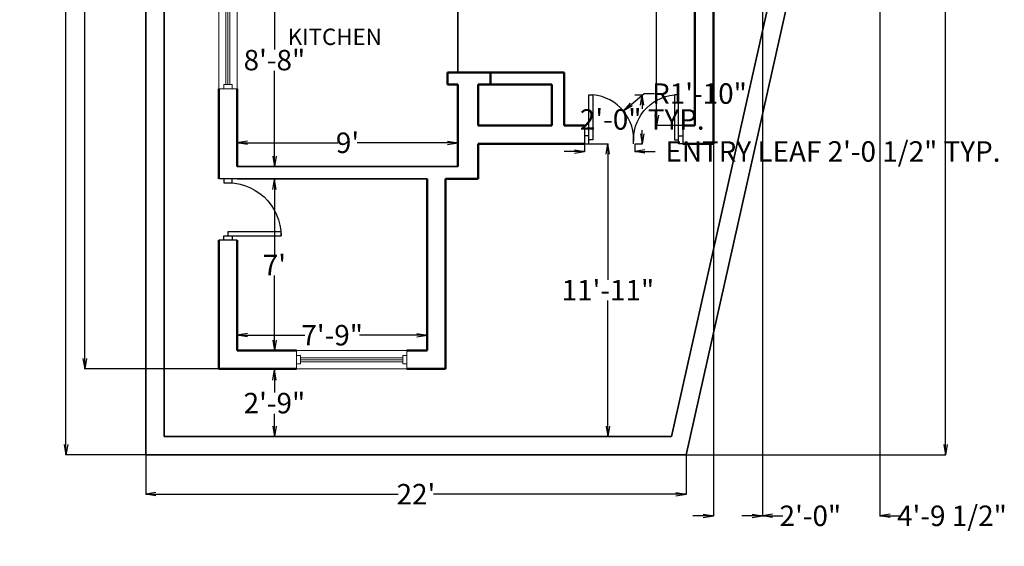
# Model space of a CAD drawing. Units: inches. Extents: x -6539 to -6057, y 19106 to 19733.
# Tile 1 of 3: x -6539 to -6057, y 19106 to 19363. Entities that reach past the tile are written whole.
import ezdxf

# ---------------------------------------------------------------- set-up
doc = ezdxf.new("R2010")
doc.units = ezdxf.units.IN
doc.header["$MEASUREMENT"] = 0
for name, color, linetype, lineweight in [('A-ANNO-DIMS', 121, 'Continuous', 18), ('A-AREA-IDEN', 250, 'Continuous', 25), ('A-WALL-EXTR', 222, 'Continuous', 50), ('C-PROP-WALL', 140, 'Continuous', 35), ('DOORS', 3, 'Continuous', 25), ('interior WALLS', 222, 'Continuous', 35), ('WINDOWS', 20, 'Continuous', 18)]:
    doc.layers.add(name, color=color, linetype=linetype, lineweight=lineweight)
doc.styles.get("Standard").update_dxf_attribs({"font": 'arial.ttf'})
doc.dimstyles.get("Standard").update_dxf_attribs({"dimtxt": 10, "dimasz": 5, "dimexe": 0.18, "dimexo": 0.0625, "dimgap": 0.09, "dimtad": 0, "dimtih": 1, "dimtoh": 1, "dimdec": 0, "dimzin": 0, "dimdsep": 46, "dimlunit": 4, "dimtxsty": 'Standard', "dimblk": 'OPEN', "dimcen": 0.09, "dimadec": 0, "dimazin": 0, "dimtfac": 1, "dimtdec": 0, "dimtofl": 0, "dimtmove": 0, "dimatfit": 0, "dimfxl": 1, "dimtolj": 1, "dimtzin": 0, "dimarcsym": 0})

# ---------------------------------------------------------------- blocks, each defined once
blk = doc.blocks.new('_Open')
at = {"color": 0, "linetype": 'ByBlock', "lineweight": -2}
for p, q in [((-1, 0.167), (0, 0)), ((-1, -0.167), (0, 0)), ((0, 0), (-1, 0))]:
    blk.add_line(p, q, dxfattribs=at)
blk = doc.blocks.new('*D3')
at = {"layer": 'A-ANNO-DIMS', "color": 0, "lineweight": -2, "transparency": 16777216}
for p, q in [((-6476.99, 19688.62), (-6516.12, 19688.62)), ((-6515.94, 19683.62), (-6515.94, 19424.78)), ((-6515.94, 19155.56), (-6515.94, 19414.39)), ((-6476.99, 19150.56), (-6516.12, 19150.56))]:
    blk.add_line(p, q, dxfattribs=at)
at = {"layer": 'Defpoints', "color": 0, "transparency": 16777216}
for p in [(-6515.94, 19688.62), (-6476.93, 19688.62), (-6476.93, 19150.56)]:
    blk.add_point(p, dxfattribs=at)
at = {"layer": 'A-ANNO-DIMS', "color": 0, "lineweight": -2, "transparency": 16777216, "xscale": 5, "yscale": 5, "zscale": 5}
for p, rotation in [((-6515.94, 19688.62), 90), ((-6515.94, 19150.56), 270)]:
    blk.add_blockref('_Open', p, dxfattribs=dict(at, rotation=rotation))
at = {"layer": 'A-ANNO-DIMS', "color": 0, "transparency": 16777216, "insert": (-6515.94, 19419.59), "char_height": 10, "attachment_point": 5}
blk.add_mtext('\\A1;44\'-10"', dxfattribs=at)
blk = doc.blocks.new('*D4')
at = {"layer": 'A-ANNO-DIMS', "color": 0, "lineweight": -2, "transparency": 16777216}
for p, q in [((-6091.64, 19688.62), (-6085.49, 19688.62)), ((-6085.67, 19683.62), (-6085.67, 19424.78)), ((-6085.67, 19155.56), (-6085.67, 19414.39)), ((-6212.44, 19150.56), (-6085.49, 19150.56))]:
    blk.add_line(p, q, dxfattribs=at)
at = {"layer": 'Defpoints', "color": 0, "transparency": 16777216}
for p in [(-6091.7, 19688.62), (-6085.67, 19688.62), (-6212.5, 19150.56)]:
    blk.add_point(p, dxfattribs=at)
at = {"layer": 'A-ANNO-DIMS', "color": 0, "lineweight": -2, "transparency": 16777216, "xscale": 5, "yscale": 5, "zscale": 5}
for p, rotation in [((-6085.67, 19688.62), 90), ((-6085.67, 19150.56), 270)]:
    blk.add_blockref('_Open', p, dxfattribs=dict(at, rotation=rotation))
at = {"layer": 'A-ANNO-DIMS', "color": 0, "transparency": 16777216, "insert": (-6085.67, 19419.59), "char_height": 10, "attachment_point": 5}
blk.add_mtext('\\A1;44\'-10"', dxfattribs=at)
blk = doc.blocks.new('*D5')
at = {"layer": 'A-ANNO-DIMS', "color": 0, "lineweight": -2, "transparency": 16777216}
for p, q in [((-6476.93, 19150.5), (-6476.93, 19131.1)), ((-6212.5, 19150.5), (-6212.5, 19131.1)), ((-6471.93, 19131.28), (-6353.37, 19131.28)), ((-6217.5, 19131.28), (-6336.05, 19131.28))]:
    blk.add_line(p, q, dxfattribs=at)
at = {"layer": 'Defpoints', "color": 0, "transparency": 16777216}
for p in [(-6476.93, 19150.56), (-6212.5, 19150.56), (-6212.5, 19131.28)]:
    blk.add_point(p, dxfattribs=at)
at = {"layer": 'A-ANNO-DIMS', "color": 0, "lineweight": -2, "transparency": 16777216, "xscale": 5, "yscale": 5, "zscale": 5, "rotation": 180}
blk.add_blockref('_Open', (-6476.93, 19131.28), dxfattribs=at)
at = {"layer": 'A-ANNO-DIMS', "color": 0, "lineweight": -2, "transparency": 16777216, "xscale": 5, "yscale": 5, "zscale": 5}
blk.add_blockref('_Open', (-6212.5, 19131.28), dxfattribs=at)
at = {"layer": 'A-ANNO-DIMS', "color": 0, "transparency": 16777216, "insert": (-6344.71, 19131.28), "char_height": 10, "attachment_point": 5}
blk.add_mtext("\\A1;22'", dxfattribs=at)
blk = doc.blocks.new('*D11')
at = {"layer": 'A-ANNO-DIMS', "color": 0, "lineweight": -2, "transparency": 16777216}
for p, q in [((-6413.44, 19395.56), (-6414.14, 19395.56)), ((-6413.96, 19390.56), (-6413.96, 19348.75)), ((-6413.96, 19296.56), (-6413.96, 19338.36)), ((-6414.02, 19291.56), (-6413.78, 19291.56))]:
    blk.add_line(p, q, dxfattribs=at)
at = {"layer": 'Defpoints', "color": 0, "transparency": 16777216}
for p in [(-6413.38, 19395.56), (-6414.08, 19291.56), (-6413.96, 19291.56)]:
    blk.add_point(p, dxfattribs=at)
at = {"layer": 'A-ANNO-DIMS', "color": 0, "lineweight": -2, "transparency": 16777216, "xscale": 5, "yscale": 5, "zscale": 5}
for p, rotation in [((-6413.96, 19395.56), 90), ((-6413.96, 19291.56), 270)]:
    blk.add_blockref('_Open', p, dxfattribs=dict(at, rotation=rotation))
at = {"layer": 'A-ANNO-DIMS', "color": 0, "transparency": 16777216, "insert": (-6413.96, 19343.56), "char_height": 10, "attachment_point": 5}
blk.add_mtext('\\A1;8\'-8"', dxfattribs=at)
blk = doc.blocks.new('*D12')
at = {"layer": 'A-ANNO-DIMS', "color": 0, "lineweight": -2, "transparency": 16777216}
for p, q in [((-6413.92, 19285.21), (-6413.78, 19285.21)), ((-6413.96, 19280.21), (-6413.96, 19248.47)), ((-6413.96, 19206.56), (-6413.96, 19238.29)), ((-6414.07, 19201.56), (-6413.78, 19201.56))]:
    blk.add_line(p, q, dxfattribs=at)
at = {"layer": 'Defpoints', "color": 0, "transparency": 16777216}
for p in [(-6413.98, 19285.21), (-6414.14, 19201.56), (-6413.96, 19201.56)]:
    blk.add_point(p, dxfattribs=at)
at = {"layer": 'A-ANNO-DIMS', "color": 0, "lineweight": -2, "transparency": 16777216, "xscale": 5, "yscale": 5, "zscale": 5}
for p, rotation in [((-6413.96, 19285.21), 90), ((-6413.96, 19201.56), 270)]:
    blk.add_blockref('_Open', p, dxfattribs=dict(at, rotation=rotation))
at = {"layer": 'A-ANNO-DIMS', "color": 0, "transparency": 16777216, "insert": (-6413.96, 19243.38), "char_height": 10, "attachment_point": 5}
blk.add_mtext("\\A1;7'", dxfattribs=at)
blk = doc.blocks.new('*D13')
at = {"layer": 'A-ANNO-DIMS', "color": 0, "lineweight": -2, "transparency": 16777216}
for p, q in [((-6413.81, 19192.09), (-6414.14, 19192.09)), ((-6413.96, 19187.09), (-6413.96, 19181.02)), ((-6413.96, 19164.56), (-6413.96, 19170.63)), ((-6414.11, 19159.56), (-6413.78, 19159.56))]:
    blk.add_line(p, q, dxfattribs=at)
at = {"layer": 'Defpoints', "color": 0, "transparency": 16777216}
for p in [(-6413.75, 19192.09), (-6414.17, 19159.56), (-6413.96, 19159.56)]:
    blk.add_point(p, dxfattribs=at)
at = {"layer": 'A-ANNO-DIMS', "color": 0, "lineweight": -2, "transparency": 16777216, "xscale": 5, "yscale": 5, "zscale": 5}
for p, rotation in [((-6413.96, 19192.09), 90), ((-6413.96, 19159.56), 270)]:
    blk.add_blockref('_Open', p, dxfattribs=dict(at, rotation=rotation))
at = {"layer": 'A-ANNO-DIMS', "color": 0, "transparency": 16777216, "insert": (-6413.96, 19175.82), "char_height": 10, "attachment_point": 5}
blk.add_mtext('\\A1;2\'-9"', dxfattribs=at)
blk = doc.blocks.new('*D14')
at = {"layer": 'A-ANNO-DIMS', "color": 0, "lineweight": -2, "transparency": 16777216}
for p, q in [((-6432.2, 19201.62), (-6432.2, 19209.2)), ((-6427.2, 19209.02), (-6399.04, 19209.02)), ((-6344.2, 19209.02), (-6372.36, 19209.02)), ((-6339.2, 19201.62), (-6339.2, 19209.2))]:
    blk.add_line(p, q, dxfattribs=at)
at = {"layer": 'Defpoints', "color": 0, "transparency": 16777216}
for p in [(-6339.2, 19209.02), (-6432.2, 19201.56), (-6339.2, 19201.56)]:
    blk.add_point(p, dxfattribs=at)
at = {"layer": 'A-ANNO-DIMS', "color": 0, "lineweight": -2, "transparency": 16777216, "xscale": 5, "yscale": 5, "zscale": 5, "rotation": 180}
blk.add_blockref('_Open', (-6432.2, 19209.02), dxfattribs=at)
at = {"layer": 'A-ANNO-DIMS', "color": 0, "lineweight": -2, "transparency": 16777216, "xscale": 5, "yscale": 5, "zscale": 5}
blk.add_blockref('_Open', (-6339.2, 19209.02), dxfattribs=at)
at = {"layer": 'A-ANNO-DIMS', "color": 0, "transparency": 16777216, "insert": (-6385.7, 19209.02), "char_height": 10, "attachment_point": 5}
blk.add_mtext('\\A1;7\'-9"', dxfattribs=at)
blk = doc.blocks.new('*D15')
at = {"layer": 'A-ANNO-DIMS', "color": 0, "lineweight": -2, "transparency": 16777216}
for p, q in [((-6432.2, 19291.62), (-6432.2, 19303.31)), ((-6427.2, 19303.13), (-6382.9, 19303.13)), ((-6329.2, 19303.13), (-6373.51, 19303.13)), ((-6324.2, 19291.62), (-6324.2, 19303.31))]:
    blk.add_line(p, q, dxfattribs=at)
at = {"layer": 'Defpoints', "color": 0, "transparency": 16777216}
for p in [(-6324.2, 19303.13), (-6432.2, 19291.56), (-6324.2, 19291.56)]:
    blk.add_point(p, dxfattribs=at)
at = {"layer": 'A-ANNO-DIMS', "color": 0, "lineweight": -2, "transparency": 16777216, "xscale": 5, "yscale": 5, "zscale": 5, "rotation": 180}
blk.add_blockref('_Open', (-6432.2, 19303.13), dxfattribs=at)
at = {"layer": 'A-ANNO-DIMS', "color": 0, "lineweight": -2, "transparency": 16777216, "xscale": 5, "yscale": 5, "zscale": 5}
blk.add_blockref('_Open', (-6324.2, 19303.13), dxfattribs=at)
at = {"layer": 'A-ANNO-DIMS', "color": 0, "transparency": 16777216, "insert": (-6378.2, 19303.13), "char_height": 10, "attachment_point": 5}
blk.add_mtext("\\A1;9'", dxfattribs=at)
blk = doc.blocks.new('*D19')
at = {"layer": 'A-ANNO-DIMS', "color": 0, "lineweight": -2, "transparency": 16777216}
for p, q in [((-6208.27, 19521.56), (-6227.12, 19521.56)), ((-6226.94, 19516.56), (-6226.94, 19421.75)), ((-6226.94, 19316.56), (-6226.94, 19411.36)), ((-6208.27, 19311.56), (-6227.12, 19311.56))]:
    blk.add_line(p, q, dxfattribs=at)
at = {"layer": 'Defpoints', "color": 0, "transparency": 16777216}
for p in [(-6226.94, 19521.56), (-6208.2, 19521.56), (-6208.2, 19311.56)]:
    blk.add_point(p, dxfattribs=at)
at = {"layer": 'A-ANNO-DIMS', "color": 0, "lineweight": -2, "transparency": 16777216, "xscale": 5, "yscale": 5, "zscale": 5}
for p, rotation in [((-6226.94, 19521.56), 90), ((-6226.94, 19311.56), 270)]:
    blk.add_blockref('_Open', p, dxfattribs=dict(at, rotation=rotation))
at = {"layer": 'A-ANNO-DIMS', "color": 0, "transparency": 16777216, "insert": (-6226.94, 19416.56), "char_height": 10, "attachment_point": 5}
blk.add_mtext('\\A1;17\'-6"', dxfattribs=at)
blk = doc.blocks.new('*D23')
at = {"layer": 'A-ANNO-DIMS', "color": 0, "lineweight": -2, "transparency": 16777216}
for p, q in [((-6261.14, 19302.56), (-6250.61, 19302.56)), ((-6250.79, 19297.56), (-6250.79, 19236.17)), ((-6250.79, 19164.56), (-6250.79, 19225.95)), ((-6258.04, 19159.56), (-6250.61, 19159.56))]:
    blk.add_line(p, q, dxfattribs=at)
at = {"layer": 'Defpoints', "color": 0, "transparency": 16777216}
for p in [(-6261.2, 19302.56), (-6258.1, 19159.56), (-6250.79, 19159.56)]:
    blk.add_point(p, dxfattribs=at)
at = {"layer": 'A-ANNO-DIMS', "color": 0, "lineweight": -2, "transparency": 16777216, "xscale": 5, "yscale": 5, "zscale": 5}
for p, rotation in [((-6250.79, 19302.56), 90), ((-6250.79, 19159.56), 270)]:
    blk.add_blockref('_Open', p, dxfattribs=dict(at, rotation=rotation))
at = {"layer": 'A-ANNO-DIMS', "color": 0, "transparency": 16777216, "insert": (-6250.79, 19231.06), "char_height": 10, "attachment_point": 5}
blk.add_mtext('\\A1;11\'-11"', dxfattribs=at)
blk = doc.blocks.new('DOOR-SWING-30IN')
for points in [[(0, 30), (0, 28), (4, 28), (4, 30)], [(2, 28), (28, 28), (28, 26), (2, 26)], [(0, 0), (0, 2), (4, 2), (4, 0)]]:
    blk.add_lwpolyline(points, close=True)
blk.add_arc((2, 28), 26, 265.5883, 0)
blk = doc.blocks.new('DOOR-ENTRY-PAIR-LEAF-24IN')
for p, q in [((0, 9), (0, 0)), ((0, 0), (2, 0))]:
    blk.add_line(p, q)
for points in [[(2, 2), (2, 24), (4, 24), (4, 2)], [(0, 0), (2, 0), (2, 4), (0, 4)]]:
    blk.add_lwpolyline(points, close=True)
blk.add_arc((2, 2), 22.09, 354.8056, 84.8056)
blk = doc.blocks.new('WIN-66IN')
for p, q in [((9, 66), (0, 66)), ((0, 66), (0, 0)), ((3.5, 64), (3.5, 2)), ((4.5, 64), (4.5, 2)), ((5.5, 64), (5.5, 2)), ((9, 66), (9, 0)), ((9, 0), (0, 0))]:
    blk.add_line(p, q)
for points in [[(2.5, 66), (2.5, 64), (6.5, 64), (6.5, 66)], [(2.5, 0), (2.5, 2), (6.5, 2), (6.5, 0)]]:
    blk.add_lwpolyline(points, close=True)
blk = doc.blocks.new('*D32')
at = {"layer": 'A-ANNO-DIMS', "color": 0, "lineweight": -2, "transparency": 16777216}
for p, q in [((-6267.2, 19298.88), (-6272.2, 19298.88)), ((-6262.2, 19302.5), (-6262.2, 19298.7)), ((-6237.67, 19302.5), (-6237.67, 19298.7)), ((-6232.67, 19298.88), (-6227.67, 19298.88))]:
    blk.add_line(p, q, dxfattribs=at)
at = {"layer": 'Defpoints', "color": 0, "transparency": 16777216}
for p in [(-6262.2, 19302.56), (-6237.67, 19302.56), (-6237.67, 19298.88)]:
    blk.add_point(p, dxfattribs=at)
at = {"layer": 'A-ANNO-DIMS', "color": 0, "lineweight": -2, "transparency": 16777216, "xscale": 5, "yscale": 5, "zscale": 5}
blk.add_blockref('_Open', (-6262.2, 19298.88), dxfattribs=at)
at = {"layer": 'A-ANNO-DIMS', "color": 0, "lineweight": -2, "transparency": 16777216, "xscale": 5, "yscale": 5, "zscale": 5, "rotation": 180}
blk.add_blockref('_Open', (-6237.67, 19298.88), dxfattribs=at)
at = {"layer": 'A-ANNO-DIMS', "color": 0, "transparency": 16777216, "insert": (-6140.69, 19298.88), "char_height": 10, "attachment_point": 5}
blk.add_mtext('\\A1;ENTRY LEAF 2\'-0 1/2" TYP.', dxfattribs=at)
blk = doc.blocks.new('*D33')
at = {"layer": 'A-ANNO-DIMS', "color": 0, "lineweight": -2, "transparency": 16777216}
for p, q in [((-6237.61, 19326.56), (-6233.81, 19326.56)), ((-6233.99, 19321.56), (-6233.99, 19319.75)), ((-6233.99, 19307.56), (-6233.99, 19309.36)), ((-6237.61, 19302.56), (-6233.81, 19302.56))]:
    blk.add_line(p, q, dxfattribs=at)
at = {"layer": 'Defpoints', "color": 0, "transparency": 16777216}
for p in [(-6237.67, 19326.56), (-6233.99, 19326.56), (-6237.67, 19302.56)]:
    blk.add_point(p, dxfattribs=at)
at = {"layer": 'A-ANNO-DIMS', "color": 0, "lineweight": -2, "transparency": 16777216, "xscale": 5, "yscale": 5, "zscale": 5}
for p, rotation in [((-6233.99, 19326.56), 90), ((-6233.99, 19302.56), 270)]:
    blk.add_blockref('_Open', p, dxfattribs=dict(at, rotation=rotation))
at = {"layer": 'A-ANNO-DIMS', "color": 0, "transparency": 16777216, "insert": (-6233.99, 19314.56), "char_height": 10, "attachment_point": 5}
blk.add_mtext('\\A1;2\'-0" TYP.', dxfattribs=at)
blk = doc.blocks.new('*D39')
at = {"layer": 'A-ANNO-DIMS', "color": 0, "lineweight": -2, "transparency": 16777216}
for p, q in [((-6441.27, 19656.56), (-6506.96, 19656.56)), ((-6506.78, 19651.56), (-6506.78, 19429.76)), ((-6506.78, 19197.56), (-6506.78, 19419.36)), ((-6441.27, 19192.56), (-6506.96, 19192.56))]:
    blk.add_line(p, q, dxfattribs=at)
at = {"layer": 'Defpoints', "color": 0, "transparency": 16777216}
for p in [(-6441.2, 19656.56), (-6506.78, 19192.56), (-6441.2, 19192.56)]:
    blk.add_point(p, dxfattribs=at)
at = {"layer": 'A-ANNO-DIMS', "color": 0, "lineweight": -2, "transparency": 16777216, "xscale": 5, "yscale": 5, "zscale": 5}
for p, rotation in [((-6506.78, 19656.56), 90), ((-6506.78, 19192.56), 270)]:
    blk.add_blockref('_Open', p, dxfattribs=dict(at, rotation=rotation))
at = {"layer": 'A-ANNO-DIMS', "color": 0, "transparency": 16777216, "insert": (-6506.78, 19424.56), "char_height": 10, "attachment_point": 5}
blk.add_mtext('\\A1;38\'-8"', dxfattribs=at)
blk = doc.blocks.new('*D40')
at = {"layer": 'A-ANNO-DIMS', "color": 0, "lineweight": -2, "transparency": 16777216}
for p, q in [((-6199.2, 19614.5), (-6199.2, 19120.53)), ((-6175.2, 19614.32), (-6175.2, 19120.53)), ((-6204.2, 19120.71), (-6209.2, 19120.71)), ((-6170.2, 19120.71), (-6165.2, 19120.71))]:
    blk.add_line(p, q, dxfattribs=at)
at = {"layer": 'Defpoints', "color": 0, "transparency": 16777216}
for p in [(-6199.2, 19614.56), (-6175.2, 19614.39), (-6175.2, 19120.71)]:
    blk.add_point(p, dxfattribs=at)
at = {"layer": 'A-ANNO-DIMS', "color": 0, "lineweight": -2, "transparency": 16777216, "xscale": 5, "yscale": 5, "zscale": 5}
blk.add_blockref('_Open', (-6199.2, 19120.71), dxfattribs=at)
at = {"layer": 'A-ANNO-DIMS', "color": 0, "lineweight": -2, "transparency": 16777216, "xscale": 5, "yscale": 5, "zscale": 5, "rotation": 180}
blk.add_blockref('_Open', (-6175.2, 19120.71), dxfattribs=at)
at = {"layer": 'A-ANNO-DIMS', "color": 0, "transparency": 16777216, "insert": (-6151.74, 19120.71), "char_height": 10, "attachment_point": 5}
blk.add_mtext('\\A1;2\'-0"', dxfattribs=at)
blk = doc.blocks.new('*D41')
at = {"layer": 'A-ANNO-DIMS', "color": 0, "lineweight": -2, "transparency": 16777216}
for p, q in [((-6175.2, 19614.32), (-6175.2, 19120.53)), ((-6117.68, 19613.92), (-6117.68, 19120.53)), ((-6180.2, 19120.71), (-6185.2, 19120.71)), ((-6112.68, 19120.71), (-6107.68, 19120.71))]:
    blk.add_line(p, q, dxfattribs=at)
at = {"layer": 'Defpoints', "color": 0, "transparency": 16777216}
for p in [(-6175.2, 19614.39), (-6117.68, 19613.98), (-6117.68, 19120.71)]:
    blk.add_point(p, dxfattribs=at)
at = {"layer": 'A-ANNO-DIMS', "color": 0, "lineweight": -2, "transparency": 16777216, "xscale": 5, "yscale": 5, "zscale": 5}
blk.add_blockref('_Open', (-6175.2, 19120.71), dxfattribs=at)
at = {"layer": 'A-ANNO-DIMS', "color": 0, "lineweight": -2, "transparency": 16777216, "xscale": 5, "yscale": 5, "zscale": 5, "rotation": 180}
blk.add_blockref('_Open', (-6117.68, 19120.71), dxfattribs=at)
at = {"layer": 'A-ANNO-DIMS', "color": 0, "transparency": 16777216, "insert": (-6082.45, 19120.71), "char_height": 10, "attachment_point": 5}
blk.add_mtext('\\A1;4\'-9 1/2"', dxfattribs=at)
blk = doc.blocks.new('*D44')
at = {"layer": 'A-ANNO-DIMS', "color": 0, "lineweight": -2, "transparency": 16777216}
for p, q in [((-6239.39, 19321.9), (-6233.05, 19327.19)), ((-6233.05, 19327.19), (-6228.05, 19327.19)), ((-6260.29, 19304.56), (-6260.11, 19304.56)), ((-6260.2, 19304.47), (-6260.2, 19304.65))]:
    blk.add_line(p, q, dxfattribs=at)
at = {"layer": 'Defpoints', "color": 0, "transparency": 16777216}
for p in [(-6243.23, 19318.7), (-6260.2, 19304.56)]:
    blk.add_point(p, dxfattribs=at)
at = {"layer": 'A-ANNO-DIMS', "color": 0, "lineweight": -2, "transparency": 16777216, "xscale": 5, "yscale": 5, "zscale": 5, "rotation": 219.8049985796428}
blk.add_blockref('_Open', (-6243.23, 19318.7), dxfattribs=at)
at = {"layer": 'A-ANNO-DIMS', "color": 0, "transparency": 16777216, "insert": (-6206, 19327.19), "char_height": 10, "attachment_point": 5}
blk.add_mtext('\\A1;R1\'-10"', dxfattribs=at)

msp = doc.modelspace()

# ---------------------------------------------------------------- linework, layer by layer
at = {"layer": 'A-WALL-EXTR'}
for p, q in [((-6208.2, 19311.56), (-6208.2, 19367.56)), ((-6199.2, 19302.56), (-6199.2, 19367.56)), ((-6314.2, 19337.56), (-6329.2, 19337.56)), ((-6329.2, 19337.56), (-6329.2, 19331.56)), ((-6314.2, 19337.56), (-6272.2, 19337.56)), ((-6308.2, 19331.56), (-6308.2, 19337.56)), ((-6272.2, 19311.56), (-6272.2, 19337.56)), ((-6441.2, 19285.56), (-6441.2, 19329.56)), ((-6441.2, 19329.56), (-6441.2, 19285.56)), ((-6432.2, 19291.56), (-6432.2, 19329.56)), ((-6329.2, 19331.56), (-6324.2, 19331.56)), ((-6324.2, 19291.56), (-6324.2, 19331.56)), ((-6314.2, 19311.56), (-6314.2, 19331.56)), ((-6314.2, 19331.56), (-6278.2, 19331.56)), ((-6314.2, 19331.56), (-6308.2, 19331.56)), ((-6278.2, 19311.56), (-6278.2, 19331.56)), ((-6314.2, 19311.56), (-6278.2, 19311.56)), ((-6272.2, 19311.56), (-6262.2, 19311.56)), ((-6214.2, 19311.56), (-6208.2, 19311.56)), ((-6314.2, 19302.56), (-6262.2, 19302.56)), ((-6314.2, 19285.56), (-6314.2, 19302.56)), ((-6214.2, 19302.56), (-6199.2, 19302.56)), ((-6339.2, 19201.56), (-6339.2, 19285.56)), ((-6330.2, 19192.56), (-6330.2, 19285.56)), ((-6330.2, 19285.56), (-6314.2, 19285.56)), ((-6441.2, 19192.56), (-6441.2, 19255.56)), ((-6441.2, 19255.56), (-6441.2, 19192.56)), ((-6432.2, 19201.56), (-6432.2, 19255.56)), ((-6432.2, 19201.56), (-6403.2, 19201.56)), ((-6349.2, 19201.56), (-6339.2, 19201.56)), ((-6441.2, 19192.56), (-6403.2, 19192.56)), ((-6349.2, 19192.56), (-6330.2, 19192.56))]:
    msp.add_line(p, q, dxfattribs=at)
at = {"layer": 'C-PROP-WALL'}
for p, q in [((-6476.93, 19688.62), (-6476.93, 19150.56)), ((-6091.7, 19688.62), (-6212.5, 19150.56)), ((-6467.93, 19679.62), (-6467.93, 19159.56)), ((-6117.68, 19613.98), (-6219.7, 19159.56)), ((-6219.7, 19159.56), (-6467.93, 19159.56)), ((-6212.5, 19150.56), (-6476.93, 19150.56))]:
    msp.add_line(p, q, dxfattribs=at)
at = {"layer": 'DOORS'}
for p, q in [((-6432.2, 19285.56), (-6441.2, 19285.56)), ((-6432.2, 19255.56), (-6441.2, 19255.56))]:
    msp.add_line(p, q, dxfattribs=at)
at = {"layer": 'interior WALLS'}
for p, q in [((-6324.2, 19337.56), (-6324.2, 19395.56)), ((-6432.2, 19291.56), (-6324.2, 19291.56)), ((-6432.2, 19285.56), (-6339.2, 19285.56))]:
    msp.add_line(p, q, dxfattribs=at)
at = {"layer": 'WINDOWS'}
for p, q in [((-6403.2, 19201.56), (-6403.2, 19192.56)), ((-6349.2, 19201.53), (-6403.2, 19201.53)), ((-6351.2, 19198.03), (-6401.2, 19198.03)), ((-6349.2, 19201.56), (-6349.2, 19192.56)), ((-6349.2, 19192.53), (-6403.2, 19192.53)), ((-6351.2, 19197.03), (-6401.2, 19197.03)), ((-6351.2, 19196.03), (-6401.2, 19196.03))]:
    msp.add_line(p, q, dxfattribs=at)
for points in [[(-6403.2, 19199.03), (-6401.2, 19199.03), (-6401.2, 19195.03), (-6403.2, 19195.03)], [(-6349.2, 19199.03), (-6351.2, 19199.03), (-6351.2, 19195.03), (-6349.2, 19195.03)]]:
    msp.add_lwpolyline(points, close=True, dxfattribs=at)

# ---------------------------------------------------------------- block references
at = {"layer": 'DOORS'}
msp.add_blockref('DOOR-ENTRY-PAIR-LEAF-24IN', (-6262.2, 19302.56), dxfattribs=at)
at = {"layer": 'DOORS', "extrusion": (0, 0, -1), "zscale": -1}
msp.add_blockref('DOOR-ENTRY-PAIR-LEAF-24IN', (6214.2, 19302.56), dxfattribs=at)
at = {"layer": 'DOORS', "extrusion": (0, 0, -1), "zscale": -1, "rotation": 180}
msp.add_blockref('DOOR-SWING-30IN', (6438.7, 19285.56), dxfattribs=at)
at = {"layer": 'WINDOWS'}
msp.add_blockref('WIN-66IN', (-6441.2, 19329.56), dxfattribs=at)

# ---------------------------------------------------------------- texts
at = {"layer": 'A-AREA-IDEN'}
msp.add_text('KITCHEN ', height=8, dxfattribs=at).set_placement((-6407.43, 19350.94))

# ---------------------------------------------------------------- dimensions: what is measured, and where the dimension line sits
at = {"layer": 'A-ANNO-DIMS'}
for base, p1, p2, override, picture, middle in [((-6515.94, 19688.62), (-6476.93, 19150.56), (-6476.93, 19688.62), {"dimclrd": 0, "dimclre": 0, "dimclrt": 0}, '*D3', (-6515.94, 19419.59)), ((-6085.67, 19688.62), (-6212.5, 19150.56), (-6091.7, 19688.62), {"dimclrd": 0, "dimclre": 0, "dimclrt": 0}, '*D4', (-6085.67, 19419.59)), ((-6506.78, 19192.56), (-6441.2, 19656.56), (-6441.2, 19192.56), {"dimdec": 1, "dimlfac": 1, "dimrnd": 0, "dimzin": 1, "dimdsep": 46, "dimlunit": 4, "dimfrac": 2}, '*D39', (-6506.78, 19424.56)), ((-6226.94, 19521.56), (-6208.2, 19311.56), (-6208.2, 19521.56), {"dimclrd": 0, "dimclre": 0, "dimclrt": 0}, '*D19', (-6226.94, 19416.56)), ((-6413.96, 19291.56), (-6413.38, 19395.56), (-6414.08, 19291.56), {"dimclrd": 0, "dimclre": 0, "dimclrt": 0, "dimtmove": 1}, '*D11', (-6413.96, 19343.56)), ((-6250.79, 19159.56), (-6261.2, 19302.56), (-6258.1, 19159.56), {"dimclrd": 0, "dimclre": 0, "dimclrt": 0}, '*D23', (-6250.79, 19231.06)), ((-6413.96, 19201.56), (-6413.98, 19285.21), (-6414.14, 19201.56), {"dimclrd": 0, "dimclre": 0, "dimclrt": 0, "dimtmove": 1}, '*D12', (-6413.96, 19243.38)), ((-6413.96, 19159.56), (-6413.75, 19192.09), (-6414.17, 19159.56), {"dimclrd": 0, "dimclre": 0, "dimclrt": 0, "dimtmove": 1}, '*D13', (-6413.96, 19175.82))]:
    dim = msp.add_linear_dim(base=base, p1=p1, p2=p2, angle=90, dimstyle='Standard', override=override, dxfattribs=at)
    dim.commit()
    dim.dimension.update_dxf_attribs({"geometry": picture, "text_midpoint": middle})
for base, p1, p2, override, picture, middle in [((-6175.2, 19120.71), (-6199.2, 19614.56), (-6175.2, 19614.39), {"dimdec": 1, "dimlfac": 1, "dimrnd": 0, "dimzin": 1, "dimdsep": 46, "dimlunit": 4, "dimfrac": 2}, '*D40', (-6151.74, 19120.71)), ((-6117.68, 19120.71), (-6175.2, 19614.39), (-6117.68, 19613.98), {"dimdec": 1, "dimlfac": 1, "dimrnd": 0, "dimzin": 1, "dimdsep": 46, "dimlunit": 4, "dimfrac": 2}, '*D41', (-6082.45, 19120.71)), ((-6324.2, 19303.13), (-6432.2, 19291.56), (-6324.2, 19291.56), {"dimclrd": 0, "dimclre": 0, "dimclrt": 0}, '*D15', (-6378.2, 19303.13)), ((-6339.2, 19209.02), (-6432.2, 19201.56), (-6339.2, 19201.56), {"dimclrd": 0, "dimclre": 0, "dimclrt": 0}, '*D14', (-6385.7, 19209.02)), ((-6212.5, 19131.28), (-6476.93, 19150.56), (-6212.5, 19150.56), {"dimclrd": 0, "dimclre": 0, "dimclrt": 0}, '*D5', (-6344.71, 19131.28))]:
    dim = msp.add_linear_dim(base=base, p1=p1, p2=p2, dimstyle='Standard', override=override, dxfattribs=at)
    dim.commit()
    dim.dimension.update_dxf_attribs({"geometry": picture, "text_midpoint": middle})
dim = msp.add_linear_dim(base=(-6237.67, 19298.88), p1=(-6262.2, 19302.56), p2=(-6237.67, 19302.56), text='ENTRY LEAF <> TYP.', dimstyle='Standard', override={"dimdec": 1, "dimlfac": 1, "dimrnd": 0, "dimzin": 1, "dimdsep": 46, "dimlunit": 4, "dimfrac": 2}, dxfattribs=at)
dim.commit()
dim.dimension.update_dxf_attribs({"geometry": '*D32', "text_midpoint": (-6140.69, 19298.88)})
dim = msp.add_radius_dim(center=(-6260.2, 19304.56), mpoint=(-6243.23, 19318.7), dimstyle='Standard', override={"dimdec": 1, "dimlfac": 1, "dimrnd": 0, "dimzin": 1, "dimdsep": 46, "dimlunit": 4, "dimfrac": 2}, dxfattribs=at)
dim.commit()
dim.dimension.update_dxf_attribs({"geometry": '*D44', "text_midpoint": (-6206, 19327.19), "dimtype": 164})
dim = msp.add_linear_dim(base=(-6233.99, 19326.56), p1=(-6237.67, 19302.56), p2=(-6237.67, 19326.56), angle=90, text='<> TYP.', dimstyle='Standard', override={"dimdec": 1, "dimlfac": 1, "dimrnd": 0, "dimzin": 1, "dimdsep": 46, "dimlunit": 4, "dimfrac": 2}, dxfattribs=at)
dim.commit()
dim.dimension.update_dxf_attribs({"geometry": '*D33', "text_midpoint": (-6233.99, 19314.56)})

doc.saveas('drawing.dxf')
